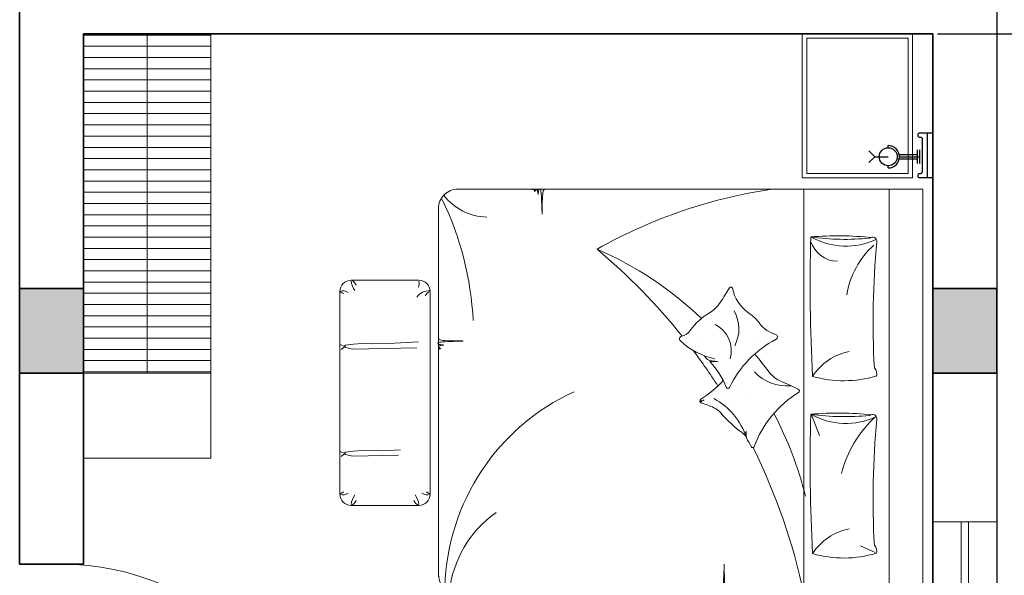
# Model space of a CAD drawing. Units: inches. Extents: x 3321 to 5237, y 11 to 1752.
# Tile 36 of 43: x 4992 to 5131, y 1478 to 1556. Entities that reach past the tile are written whole.
import ezdxf

# ---------------------------------------------------------------- set-up
doc = ezdxf.new("R2010")
doc.units = ezdxf.units.IN
for name, color, linetype, lineweight in [('A-ANNO-DIMS', 2, 'Continuous', 18), ('A-COLS', 1, 'Continuous', 35), ('A-DOOR', 4, 'Continuous', 18), ('A-FLOR-CASE', 8, 'Continuous', 18), ('A-FLOR-CASE-PATT', 8, 'Continuous', 13), ('A-FLOR-EDGE', 7, 'Continuous', 25), ('A-GLAZ', 5, 'Continuous', 18), ('A-WALL', 7, 'Continuous', 35), ('FUR', 42, 'Continuous', 18)]:
    doc.layers.add(name, color=color, linetype=linetype, lineweight=lineweight)
for name, color, linetype in [('CEIL', 4, 'Continuous'), ('ELEC', 4, 'Continuous'), ('wood', 26, 'Continuous')]:
    doc.layers.add(name, color=color, linetype=linetype)
doc.styles.get("Standard").update_dxf_attribs({"font": 'arial.ttf'})
doc.dimstyles.new('ISO-25', dxfattribs={"dimtxt": 9, "dimasz": 2.5, "dimexe": 1.25, "dimexo": 0.625, "dimtad": 1, "dimdec": 1, "dimlunit": 3, "dimtxsty": 'Standard', "dimcen": 2.5, "dimclrd": 4, "dimclre": 4, "dimclrt": 256, "dimadec": 0, "dimazin": 0, "dimtfac": 1, "dimtdec": 1, "dimtmove": 0, "dimatfit": 3, "dimfxl": 1, "dimarcsym": 0})

# ---------------------------------------------------------------- blocks, each defined once
blk = doc.blocks.new('*U4')
for p, q in [((0, 0), (0, -6)), ((-36, 0), (-36, -6))]:
    blk.add_line(p, q)
blk.add_lwpolyline([(0, 0), (0, 36), (-1.75, 36), (-1.75, 0)], close=True)
blk.add_arc((0, 0), 36, 90, 180)
blk = doc.blocks.new('*X127')
at = {"color": 0}
for p, q in [((3155.9, 8182.9), (3155.9, 8182.9)), ((3147.8, 8143.4), (3147.8, 8143.4)), ((3283, 8049.6), (3283, 8049.6)), ((3209.5, 8023.9), (3209.5, 8023.9)), ((3251.6, 7997), (3251.6, 7997)), ((3154.1, 7950.7), (3154.1, 7950.7))]:
    blk.add_line(p, q, dxfattribs=at)
blk = doc.blocks.new('*X126')
at = {"color": 0}
for p, q in [((3155.9, 8182.9), (3155.9, 8182.9)), ((3139.8, 7939.7), (3139.8, 7939.7))]:
    blk.add_line(p, q, dxfattribs=at)
blk = doc.blocks.new('*X125')
at = {"color": 0}
for p, q in [((3155.9, 8182.9), (3155.9, 8182.9)), ((3139.8, 7939.7), (3139.8, 7939.7))]:
    blk.add_line(p, q, dxfattribs=at)
blk = doc.blocks.new('*X124')
at = {"color": 0}
for p, q in [((3163, 7776.2), (3163, 7776.2)), ((3422.2, 7761.3), (3422.2, 7761.3)), ((3244.3, 7698.6), (3244.3, 7698.6)), ((3236.2, 7675.7), (3236.2, 7675.7)), ((3340.3, 7689.4), (3340.3, 7689.4))]:
    blk.add_line(p, q, dxfattribs=at)
blk = doc.blocks.new('BED1')
for p, q in [((0, -1000), (0, 800)), ((150, 800), (0, 800)), ((150, 800), (150, -1000)), ((2058.7, 800), (150, 800)), ((528, 800), (528, -1000)), ((211.8, 614.9), (277.5, 585.4)), ((2537.2, 404.9), (2237.2, 404.9)), ((2187.2, 354.9), (2187.2, -545.1)), ((2587.2, -545.1), (2587.2, 354.9)), ((2566.3, 178.5), (2565.2, 177.4)), ((2582, 188.1), (2565.4, 174.8)), ((2565.4, 174.8), (2585.7, 165.4)), ((2566.3, -296.8), (2565.2, -297.9)), ((2582, -287.1), (2565.4, -300.5)), ((2565.4, -300.5), (2585.7, -309.9)), ((2237.2, -595.1), (2537.2, -595.1)), ((150, -1000), (0, -1000)), ((150, -1000), (2063.5, -1000))]:
    blk.add_line(p, q)
for points in [[(934, 797.9), (930.9, 797.7), (928.3, 797.4), (926.3, 796.9), (924.9, 796.3), (923.8, 795.6), (923.1, 794.8), (922.7, 793.8), (922.5, 792.7), (922.4, 791.5), (922.5, 790.3), (922.6, 789.2), (922.6, 788.3), (922.6, 787.6), (922.4, 787.3), (922, 787.4), (921.4, 787.9), (920.6, 788.9), (919.5, 790.2), (918.4, 791.6), (917.1, 793.1), (915.9, 794.6), (914.6, 796), (913.3, 797.1), (912.2, 797.9), (911.1, 798.3), (910.1, 798.4), (909.2, 798), (908.3, 797.1), (907.5, 795.8), (906.8, 793.9), (906, 791.4), (905.4, 788.5), (904.8, 785.2), (904.2, 781.7), (903.7, 778.4), (903.2, 775.4), (902.8, 772.9), (902.5, 771.3), (902.3, 770.6), (902.1, 771.2), (902, 772.8), (901.8, 775.2), (901.7, 778.1), (901.5, 781.5), (901.2, 785), (900.8, 788.4), (900.2, 791.5), (899.5, 794.1), (898.6, 796.2), (897.6, 797.9), (896.5, 799.2), (895.3, 800), (894.1, 800.5), (893, 800.7), (891.9, 800.5), (890.9, 800.1), (890, 799), (889.1, 797.1), (888.3, 794), (887.6, 789.3), (886.9, 782.9), (886.2, 774.2), (885.5, 763.1), (884.8, 749.5), (884.2, 734.2), (883.6, 718.3), (883, 702.8), (882.5, 688.8), (882, 677.5), (881.7, 669.8), (881.5, 666.9), (881.3, 669.4), (881.3, 676.7), (881.3, 687.8), (881.2, 701.5), (881.1, 716.8), (880.8, 732.6), (880.2, 748), (879.4, 761.8), (878.3, 773.2), (876.9, 782.2), (875.1, 789.2), (872.9, 794.4), (870.3, 798), (869, 799)], [(2150, -913.5), (2150, 723.2)], [(2327.6, 182.3), (2530, 185.9), (2550.8, 181.9), (2561.7, 179), (2566, 176.7), (2566.9, 174.4), (2566.3, 171.9), (2562, 169.2), (2550.3, 166.5), (2527.7, 163.9), (2490.6, 161.8), (2345.5, 160.2), (2317.8, 158.5)], [(494.7, 3.1), (458.9, 95.3)], [(2149.7, -259.9), (2150, -268.4), (2150.1, -274.1), (2150.1, -278.1), (2150, -281.4), (2149.8, -284), (2149.5, -286.1), (2149.1, -287.8), (2148.7, -289), (2148.1, -289.9), (2147.4, -290.5), (2146.6, -290.8), (2145.6, -291), (2144.6, -291), (2143.6, -291), (2142.7, -290.9), (2141.9, -290.9), (2141.4, -290.9), (2141.1, -291), (2141.2, -291.4), (2141.7, -291.9), (2142.5, -292.6), (2143.5, -293.4), (2144.7, -294.4), (2146, -295.4), (2147.2, -296.5), (2148.4, -297.6), (2149.3, -298.6), (2150, -299.6), (2150.3, -300.5), (2150.4, -301.3), (2150, -302.1), (2149.3, -302.8), (2148.2, -303.5), (2146.6, -304.1), (2144.6, -304.7), (2142.1, -305.2), (2139.3, -305.7), (2136.5, -306.2), (2133.7, -306.6), (2131.2, -307), (2129.2, -307.3), (2127.8, -307.6), (2127.3, -307.8), (2127.7, -308), (2129, -308.1), (2131, -308.2), (2133.5, -308.3), (2136.3, -308.5), (2139.2, -308.7), (2142, -309), (2144.6, -309.5), (2146.8, -310.1), (2148.6, -310.9), (2150, -311.7), (2151, -312.7), (2151.7, -313.6), (2152.1, -314.6), (2152.3, -315.6), (2152.2, -316.5), (2151.8, -317.3), (2150.9, -318.1), (2149.3, -318.8), (2146.7, -319.4), (2142.8, -320), (2137.4, -320.6), (2130.2, -321.2), (2121, -321.8), (2109.7, -322.3), (2096.9, -322.9), (2083.6, -323.4), (2070.7, -323.9), (2059.1, -324.3), (2049.6, -324.7), (2043.2, -325), (2040.8, -325.2), (2042.9, -325.3), (2049, -325.3), (2058.2, -325.3), (2069.6, -325.4), (2082.3, -325.5), (2095.6, -325.8), (2108.4, -326.2), (2119.9, -326.8), (2129.4, -327.8), (2136.9, -329), (2142.7, -330.5), (2147, -332.3), (2150, -334.4), (2150.9, -335.6)], [(2246.5, -294.4), (2530, -289.4), (2550.8, -293.4), (2561.7, -296.3), (2566, -298.6), (2566.9, -300.8), (2566.3, -303.4), (2562, -306.1), (2550.3, -308.8), (2527.7, -311.3), (2490.6, -313.5), (2345.5, -315), (2238.6, -321.8)], [(1733.7, -998.3), (1731.1, -998.1), (1729, -997.8), (1727.4, -997.4), (1726.1, -997), (1725.2, -996.4), (1724.7, -995.7), (1724.3, -994.8), (1724.1, -993.9), (1724.1, -992.9), (1724.1, -991.9), (1724.2, -991), (1724.2, -990.2), (1724.2, -989.7), (1724.1, -989.4), (1723.8, -989.5), (1723.2, -990), (1722.5, -990.8), (1721.7, -991.8), (1720.7, -993), (1719.7, -994.3), (1718.6, -995.5), (1717.5, -996.6), (1716.5, -997.6), (1715.5, -998.3), (1714.6, -998.6), (1713.8, -998.6), (1713, -998.3), (1712.3, -997.6), (1711.7, -996.5), (1711, -994.9), (1710.4, -992.9), (1709.9, -990.4), (1709.4, -987.6), (1708.9, -984.8), (1708.5, -982), (1708.1, -979.5), (1707.8, -977.4), (1707.5, -976.1), (1707.3, -975.5), (1707.1, -976), (1707, -977.3), (1706.9, -979.3), (1706.8, -981.8), (1706.7, -984.6), (1706.4, -987.5), (1706.1, -990.3), (1705.6, -992.9), (1705, -995.1), (1704.2, -996.9), (1703.4, -998.3), (1702.4, -999.3), (1701.5, -1000), (1700.5, -1000.4), (1699.6, -1000.6), (1698.7, -1000.4), (1697.8, -1000.1), (1697, -999.2), (1696.3, -997.6), (1695.7, -995), (1695.1, -991.1), (1694.5, -985.7), (1693.9, -978.5), (1693.3, -969.3), (1692.8, -957.9), (1692.2, -945.2), (1691.7, -931.9), (1691.2, -919), (1690.8, -907.4), (1690.4, -897.9), (1690.1, -891.5), (1689.9, -889.1), (1689.8, -891.2), (1689.8, -897.3), (1689.8, -906.5), (1689.7, -917.9), (1689.6, -930.6), (1689.4, -943.8), (1688.9, -956.6), (1688.3, -968.1), (1687.3, -977.6), (1686.1, -985.2), (1684.6, -991), (1682.8, -995.3), (1680.7, -998.3), (1679.6, -999.2)]]:
    blk.add_lwpolyline(points)
for points in [[(205.5, 619.6, 0.267769), (215.1, 582.4, -0.037739), (204.3, 21.8, 0.684696), (236.7, 5.5, -0.060702), (497.2, 0.1, -0.046649), (225.9, 3.1, -1.318436)], [(489.2, 619.6, 0.144019), (207.6, 617.9, 0.248643)], [(497.2, 0.1, 0.021276), (489.2, 619.6, -0.206383), (326.6, 509.4, 0.237198)], [(211.8, 12.8, 0.143972), (361.6, 262.9, 1.292232)], [(886.4, -150, -0.069098), (985, -66.5, 0.658965), (982.1, -48.7, -0.049789), (927.4, -29, -0.103757), (896.6, -5.4, 0.055725), (800.9, 83.3, -0.11866), (782.7, 104.9, 0.016811), (761.6, 143.9, 0.70791), (748.3, 144, -0.16964), (551.9, -96.6, 0.664036), (554, -110.7, 0.023706), (627, -144.7, -0.134834), (683.2, -188, 0.012748), (746.3, -267.4)], [(969.1, -259.1, 0.263265), (936.3, -236.9, -0.026108), (909.2, -233.2, 0.027613), (945.1, -234.2, -0.089259), (872.7, -120, 0.662242), (857.6, -119.3, -0.162037), (651.8, -332.7, 0.676499), (654, -354.5, -0.160513), (722.9, -401.5, 0.07473), (773.5, -450.3, -0.187721), (845.5, -559.9, 0.70791), (858.8, -561.4, -0.010003), (898.6, -497.3, -0.113819), (947.3, -450.2, 0.099539), (1032.5, -372.4, -0.173425), (1070.9, -346.4, 0.589988), (1076.2, -326.1, 0.137312), (923.9, -245.9, 0.137312)], [(205.5, -168.2, 0.267769), (215.1, -205.4, -0.037739), (204.3, -766, 0.684696), (236.7, -782.3, -0.060702), (497.2, -787.7, -0.046649), (225.9, -784.7, -1.318436)], [(489.2, -168.2, 0.144019), (207.6, -169.9, 0.248643)], [(497.2, -787.7, 0.021276), (489.2, -168.2, -0.206383), (326.6, -278.4, 0.237198)], [(1446, -733.4, -0.095039), (652.8, -1001.7)]]:
    blk.add_lwpolyline(points, format="xyb")
for centre, radius, start, end in [((3208.8, 1363.3), 2739.4, 191.8679, 206.3247), ((1608.1, 842.5), 496.3, 305.1901, 354.0206), ((2062.7, 713.7), 86.5, 0, 93.5376), ((1138.6, 793.9), 983.2, 294.6078, 358.3033), ((2237.2, 354.9), 50, 90, 180), ((2321.1, 409.7), 84.5, 185.6196, 217.1396), ((2227.5, 373.5), 32.8, 17.833, 72.8005), ((2546.9, 373.5), 32.8, 107.1995, 162.167), ((2453.3, 409.7), 84.5, 322.8604, 354.3804), ((2537.2, 354.9), 50, 0, 90), ((2098.7, 754.7), 1625, 193.905, 207.8169), ((2201.9, 323.3), 34.8, 50.8413, 114.9586), ((2212.2, 381.5), 36.5, 226.8095, 258.3841), ((2572.5, 323.3), 34.8, 65.0414, 129.1587), ((2562.2, 381.5), 36.5, 281.6159, 313.1905), ((751.8, 88.7), 34.9, 336.8352, 27.7218), ((684.2, 86), 100.3, 353.675, 10.882), ((1074.1, 198.8), 306.1, 197.8602, 241.5122), ((341.4, -277.7), 318.5, 60.7125, 115.009), ((983.7, -79.5), 20.8, 73.7967, 130.4566), ((978.5, -68.6), 14.3, 39.7097, 85.9506), ((602.5, -324), 198.6, 43.2035, 95.0556), ((3208.8, 1363.3), 2739.4, 212.9314, 216.951), ((981.1, -281.8), 131.1, 164.0372, 243.4536), ((980, -379), 163.4, 152.6104, 209.361), ((3208.8, 1363.3), 2739.4, 218.6329, 229.9449), ((2098.7, 754.7), 1625, 226.5887, 246.3156), ((3402.5, -342.9), 1408.5, 182.9917, 205.6819), ((2188.1, -476.2), 73, 269.4513, 322.8027), ((-34.4, -471.2), 376.5, 312.0118, 350.9635), ((2178, -513.5), 33, 286.1827, 338.1386), ((2237.2, -545.1), 50, 180, 270), ((2271.1, -580.9), 35.8, 148.9055, 197.5541), ((2453.3, -600), 84.5, 5.6196, 37.1396), ((2537.2, -545.1), 50, 270, 0), ((2572.5, -513.6), 34.8, 230.8413, 294.9586), ((2562.2, -571.8), 36.5, 46.8095, 78.3841), ((2546.9, -563.8), 32.8, 197.833, 252.8005), ((375.7, -807.4), 128.2, 17.4073, 88.5129), ((341.4, -1065.5), 318.5, 60.7125, 115.009), ((1929.1, -1126), 250.5, 37.8553, 88.4405), ((2063.5, -913.5), 86.5, 270, 0)]:
    blk.add_arc(centre, radius, start, end)
for name in ['*X126', '*X125', '*X127', '*X124']:
    blk.add_blockref(name, (-2425.3, -8101.4))
blk = doc.blocks.new('APLIQ')
at = {"layer": 'ELEC'}
for p, q in [((0, 0.2), (-0.0261, 0.2261)), ((0, 0.2), (0.0261, 0.2261)), ((0, 0.2), (0, 0.14)), ((-0.05, 0.14), (-0.04, 0.14)), ((0.04, 0.14), (0.05, 0.14)), ((-0.01, 0.09), (-0.01, 0.01)), ((0, 0.09), (0, 0)), ((0.01, 0.09), (0.01, 0.01)), ((-0.03, 0.01), (0.03, 0.01)), ((-0.03, 0), (0.03, 0))]:
    blk.add_line(p, q, dxfattribs=at)
blk.add_circle((0, 0.14), 0.04, dxfattribs=at)
blk.add_arc((0, 0.14), 0.05, 180, 0, dxfattribs=at)
blk = doc.blocks.new('A$C68AE1801')
at = {"layer": 'FUR'}
for points in [[(2.5416, 3.18), (2.5416, 2.54), (2.0516, 2.54), (2.0516, 3.18)], [(2.5216, 3.16), (2.5216, 2.56), (2.0716, 2.56), (2.0716, 3.16)], [(2.5416, 0), (2.5416, 0.64), (2.0516, 0.64), (2.0516, 0)], [(2.5216, 0.02), (2.5216, 0.62), (2.0716, 0.62), (2.0716, 0.02)]]:
    blk.add_lwpolyline(points, close=True, dxfattribs=at)
at = {"layer": 'wood'}
for p, q in [((2.6057, 2.74), (2.6057, 2.54)), ((2.6057, 0.44), (2.6057, 0.64))]:
    blk.add_line(p, q, dxfattribs=at)
for points in [[(2.5657, 2.728), (2.5657, 2.732, -0.414214), (2.5737, 2.74), (2.6321, 2.74), (2.6321, 2.54), (2.5737, 2.54, -0.414214), (2.5657, 2.548), (2.5657, 2.552, -0.414214), (2.5737, 2.56), (2.5777, 2.56, 0.414214), (2.5857, 2.568), (2.5857, 2.712, 0.414214), (2.5777, 2.72), (2.5737, 2.72, -0.414214)], [(2.5657, 0.452), (2.5657, 0.448, 0.414214), (2.5737, 0.44), (2.6321, 0.44), (2.6321, 0.64), (2.5737, 0.64, 0.414214), (2.5657, 0.632), (2.5657, 0.628, 0.414214), (2.5737, 0.62), (2.5777, 0.62, -0.414214), (2.5857, 0.612), (2.5857, 0.468, -0.414214), (2.5777, 0.46), (2.5737, 0.46, 0.414214)]]:
    blk.add_lwpolyline(points, format="xyb", close=True, dxfattribs=at)
at = {"layer": 'CEIL', "rotation": 90}
blk.add_blockref('APLIQ', (2.5736, 2.634), dxfattribs=at)
at = {"layer": 'CEIL', "xscale": -1, "rotation": 90}
blk.add_blockref('APLIQ', (2.5736, 0.546), dxfattribs=at)
at = {"layer": 'FUR', "xscale": 0.001, "yscale": 0.001, "zscale": 0.001, "rotation": 180}
blk.add_blockref('BED1', (2.5872, 1.49), dxfattribs=at)
blk = doc.blocks.new('COL-9X12-FURN-PLAN')
h = blk.add_hatch(color=256)
h.dxf.hatch_style = 1
h.paths.add_polyline_path([(0, 12), (0, 0), (9, 0), (9, 12)])
blk.add_lwpolyline([(0, 0), (9, 0), (9, 12), (0, 12)], close=True)
blk = doc.blocks.new('WIN-48IN-9IN-WALL')
for p, q in [((0, 0), (0, 9)), ((48, 0), (48, 9)), ((0, 5), (48, 5)), ((0, 4), (48, 4))]:
    blk.add_line(p, q)
blk = doc.blocks.new('*D193')
at = {"layer": 'A-ANNO-DIMS', "color": 4, "lineweight": -2, "transparency": 16777216}
for p, q in [((5136.26, 1554.34), (5136.26, 1691.49)), ((5121.71, 1554.34), (5137.51, 1554.34)), ((5136.26, 1455.64), (5136.26, 1551.84)), ((5121.71, 1453.14), (5137.51, 1453.14))]:
    blk.add_line(p, q, dxfattribs=at)
at = {"layer": 'A-ANNO-DIMS', "color": 4, "transparency": 16777216}
for points in [[(5135.85, 1551.84), (5136.68, 1551.84), (5136.26, 1554.34)], [(5135.85, 1455.64), (5136.68, 1455.64), (5136.26, 1453.14)]]:
    blk.add_solid(points, dxfattribs=at)
at = {"layer": 'Defpoints', "color": 0, "transparency": 16777216}
for p in [(5121.08, 1554.34), (5136.26, 1554.34), (5121.08, 1453.14)]:
    blk.add_point(p, dxfattribs=at)
at = {"layer": 'A-ANNO-DIMS', "transparency": 16777216, "insert": (5130.98, 1624.17), "char_height": 9, "attachment_point": 5, "rotation": 90}
blk.add_mtext('BED GROUP 8\'-5" TYP.', dxfattribs=at)

msp = doc.modelspace()

# ---------------------------------------------------------------- hatches: boundary and pattern name
at = {"layer": 'A-FLOR-CASE-PATT'}
h = msp.add_hatch(dxfattribs=at)
h.set_pattern_fill('ANSI31', color=256, scale=0.5, angle=135)
h.set_pattern_definition([(180, (-1652.0904, 0), (-1e-16, -1.5875), [])])
h.paths.add_polyline_path([(5001.08, 1506.34), (5019.08, 1506.34), (5019.08, 1554.34), (5001.08, 1554.34)])

# ---------------------------------------------------------------- linework, layer by layer
at = {"layer": 'A-FLOR-CASE'}
for p, q in [((5010.08, 1506.34), (5010.08, 1554.34)), ((5019.08, 1554.34), (5019.08, 1494.34)), ((5001.08, 1506.34), (5019.08, 1506.34)), ((5001.08, 1494.34), (5019.08, 1494.34))]:
    msp.add_line(p, q, dxfattribs=at)
at = {"layer": 'A-FLOR-EDGE'}
msp.add_line((5130.08, 1687.34), (5130.08, 1091.34), dxfattribs=at)
at = {"layer": 'A-WALL'}
for p, q in [((4992.08, 1558.34), (4992.08, 1479.34)), ((5001.08, 1554.34), (5001.08, 1479.34)), ((5001.08, 1554.34), (5121.08, 1554.34)), ((5121.08, 1554.34), (5121.08, 1434.34)), ((4992.08, 1518.34), (5001.08, 1518.34)), ((4992.08, 1479.34), (5001.08, 1479.34))]:
    msp.add_line(p, q, dxfattribs=at)

# ---------------------------------------------------------------- block references
at = {"layer": 'A-COLS'}
for p in [(4992.08, 1506.34), (5121.08, 1506.34)]:
    msp.add_blockref('COL-9X12-FURN-PLAN', p, dxfattribs=at)
at = {"layer": 'A-DOOR', "rotation": 270}
msp.add_blockref('*U4', (4998.08, 1443.34), dxfattribs=at)
at = {"layer": 'A-GLAZ', "rotation": 90.00000000000043}
msp.add_blockref('WIN-48IN-9IN-WALL', (5130.08, 1437.34), dxfattribs=at)
at = {"layer": 'FUR', "xscale": 31.82298296329056, "yscale": 31.82298296329056, "zscale": 31.82298296329056}
msp.add_blockref('A$C68AE1801', (5037.32, 1453.14), dxfattribs=at)

# ---------------------------------------------------------------- dimensions: what is measured, and where the dimension line sits
at = {"layer": 'A-ANNO-DIMS'}
dim = msp.add_linear_dim(base=(5136.26, 1554.34), p1=(5121.08, 1453.14), p2=(5121.08, 1554.34), angle=90, text='BED GROUP <> TYP.', dimstyle='ISO-25', override={"dimdec": 1, "dimlfac": 1, "dimrnd": 0, "dimzin": 1, "dimdsep": 46, "dimlunit": 4, "dimfrac": 2}, dxfattribs=at)
dim.commit()
dim.dimension.update_dxf_attribs({"geometry": '*D193', "text_midpoint": (5130.98, 1624.17)})

doc.saveas('drawing.dxf')
